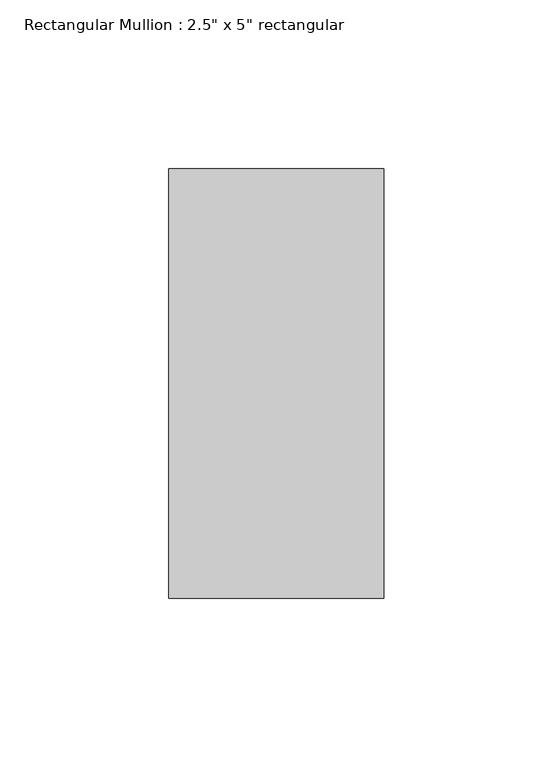
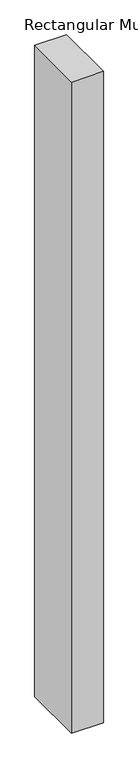
"""IFC4 building model written with IfcOpenShell, lengths in millimetres: member geometry."""

from ifc_helpers import new_model, si_unit, frame, origin, place, context, project, spatial, polyline, outline, extrude, source, transform, mapped, element, save


def member_c6627131(model_context):
    return source(origin(), model_context, "Body", "SweptSolid", [
        extrude(outline(polyline([(0.0, 63.5), (0.0, -63.5), (-63.5, -63.5), (-63.5, 63.5), (0.0, 63.5)])), frame((0.0, 0.0, -1371.6), z_axis=(0.0, 0.0, 1.0), x_axis=(1.0, 0.0, 0.0)), (0.0, 0.0, 1.0), 1371.6),
    ])


if __name__ == "__main__":
    model = new_model("IFC4")
    model_context = context("Model", 3, world=origin())
    ifc_project = project(units=[si_unit("LENGTHUNIT", "METRE", prefix="MILLI")], contexts=[model_context])
    site = spatial("IfcSite", under=ifc_project)
    building = spatial("IfcBuilding", under=site)
    placement = place(None, origin())
    member_shape = member_c6627131(model_context)
    element("IfcMember", 1, ObjectType="Rectangular Mullion : 2.5\" x 5\" rectangular", at=placement, inside=building, context=model_context, shape_type="MappedRepresentation", body=[
        mapped(member_shape, transform((0.0, 0.0, 0.0), x_axis=(1.0, 0.0, 0.0), y_axis=(0.0, 1.0, 0.0), z_axis=(0.0, 0.0, 1.0))),
    ])
    save(model, "model.ifc")

# Revit data of these elements
# Type "Rectangular Mullion : 2.5\" x 5\" rectangular"
#   built-in parameter 1007304 = 0.416667 (stored number, unit not read)
#   built-in parameter 1007301 = 0.104167 (stored number, unit not read)
#   built-in parameter 1007300 = 0.104167 (stored number, unit not read)
# Element 1 (IfcMember, "Rectangular Mullion : 2.5\" x 5\" rectangular")
#   Materials on its faces: "Aluminum"
# Materials
#   "Aluminum": class "Metal", colour RGB 247 247 247, transparency 0, Description = "Aluminum 6061", Cost = 0
